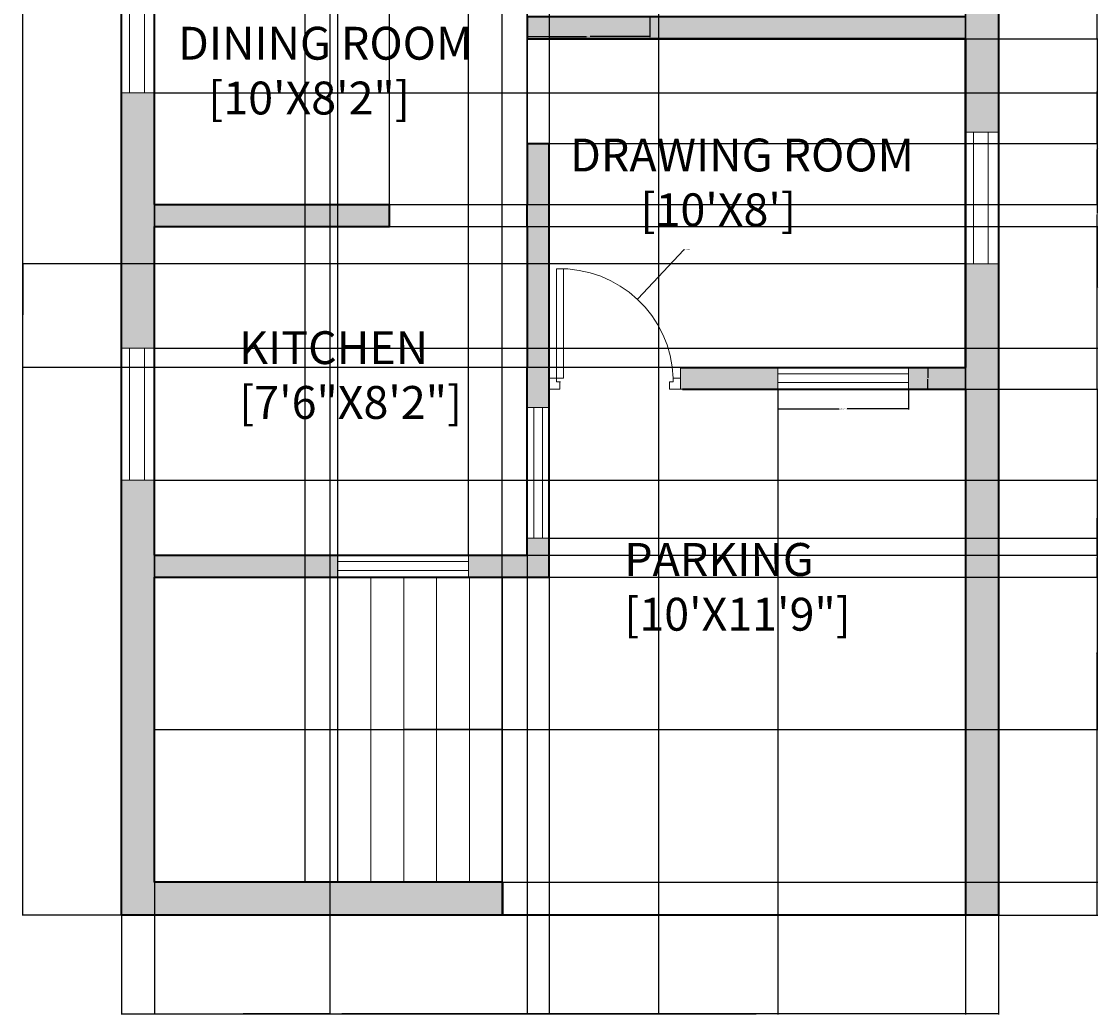
# Model space of a CAD drawing. Units: inches. Extents: x 1963 to 2258, y 1522 to 2116.
# Tile 1 of 3: x 1963 to 2258, y 1522 to 1793. Entities that reach past the tile are written whole.
import ezdxf

# ---------------------------------------------------------------- set-up
doc = ezdxf.new("R2010")
doc.units = ezdxf.units.IN
for name, color, linetype, lineweight in [('A-ANNO-DIMS', 2, 'Continuous', 18), ('A-AREA-IDEN', 7, 'Continuous', 18), ('A-DOOR', 3, 'Continuous', 18), ('A-FLOR-STRS', 7, 'Continuous', 18), ('A-GLAZ', 4, 'Continuous', 18), ('A-WALL', 7, 'Continuous', 35), ('A-WALL-PATT', 250, 'Continuous', 13)]:
    doc.layers.add(name, color=color, linetype=linetype, lineweight=lineweight)
doc.styles.get("Standard").update_dxf_attribs({"font": 'arial.ttf'})
doc.dimstyles.get("Standard").update_dxf_attribs({"dimtxt": 0.18, "dimasz": 0.18, "dimexe": 0.18, "dimexo": 0.0625, "dimgap": 0.09, "dimtad": 0, "dimtih": 1, "dimtoh": 1, "dimdec": 4, "dimzin": 0, "dimdsep": 46, "dimtxsty": 'Standard', "dimcen": 0.09, "dimadec": 0, "dimazin": 0, "dimtfac": 1, "dimtdec": 4, "dimtofl": 0, "dimtmove": 0, "dimatfit": 3, "dimfxl": 1, "dimtolj": 1, "dimtzin": 0, "dimarcsym": 0})

# ---------------------------------------------------------------- blocks, each defined once
blk = doc.blocks.new('WIN-36-9IN-WALL')
for p, q in [((-9, 0), (-9, 36.12)), ((-9, 36.12), (0, 36.12)), ((-6.81, 0), (-6.81, 36.12)), ((-4.5, 36.12), (-2.78, 36.12)), ((-2.78, 36.12), (-2.78, 0)), ((0, 36.12), (0, 0)), ((0, 0), (-9, 0)), ((-2.78, 0), (-6.81, 0)), ((0, 0), (-4.5, 0))]:
    blk.add_line(p, q)
blk = doc.blocks.new('WIN-36-6IN-WALL')
for p, q in [((35.74, 5.97), (0, 5.97)), ((0, 5.97), (0, 0)), ((35.74, 0), (35.74, 5.97)), ((0, 1.82), (0, 4.22)), ((0, 4.22), (35.74, 4.22)), ((0, 0), (0, 2.99)), ((35.74, 2.99), (35.74, 4.22)), ((35.74, 4.22), (35.74, 1.82)), ((35.74, 1.82), (0, 1.82)), ((0, 0), (35.74, 0))]:
    blk.add_line(p, q)
blk = doc.blocks.new('*D8')
at = {"layer": 'A-ANNO-DIMS', "color": 0, "lineweight": -2, "transparency": 16777216}
for p, q in [((2169.76, 1692.68), (2169.76, 1687.21)), ((2205.49, 1692.68), (2205.49, 1687.21)), ((2169.94, 1687.39), (2186.51, 1687.39)), ((2205.31, 1687.39), (2188.74, 1687.39))]:
    blk.add_line(p, q, dxfattribs=at)
at = {"layer": 'A-ANNO-DIMS', "color": 0, "transparency": 16777216}
for points in [[(2169.94, 1687.42), (2169.94, 1687.36), (2169.76, 1687.39)], [(2205.31, 1687.42), (2205.31, 1687.36), (2205.49, 1687.39)]]:
    blk.add_solid(points, dxfattribs=at)
at = {"layer": 'Defpoints', "color": 0, "transparency": 16777216}
for p in [(2169.76, 1692.75), (2205.49, 1692.75), (2205.49, 1687.39)]:
    blk.add_point(p, dxfattribs=at)
at = {"layer": 'A-ANNO-DIMS', "color": 0, "transparency": 16777216, "insert": (2187.62, 1687.39), "char_height": 0.18, "attachment_point": 5}
blk.add_mtext('\\A1;WINDOW 36 TYP.', dxfattribs=at)
blk = doc.blocks.new('*D9')
at = {"layer": 'A-ANNO-DIMS', "color": 0, "lineweight": -2, "transparency": 16777216}
for p, q in [((2205.56, 1698.72), (2211.03, 1698.72)), ((2210.85, 1698.54), (2210.85, 1695.92)), ((2210.85, 1692.93), (2210.85, 1695.55)), ((2205.56, 1692.75), (2211.03, 1692.75))]:
    blk.add_line(p, q, dxfattribs=at)
at = {"layer": 'A-ANNO-DIMS', "color": 0, "transparency": 16777216}
for points in [[(2210.82, 1698.54), (2210.88, 1698.54), (2210.85, 1698.72)], [(2210.82, 1692.93), (2210.88, 1692.93), (2210.85, 1692.75)]]:
    blk.add_solid(points, dxfattribs=at)
at = {"layer": 'Defpoints', "color": 0, "transparency": 16777216}
for p in [(2205.49, 1698.72), (2210.85, 1698.72), (2205.49, 1692.75)]:
    blk.add_point(p, dxfattribs=at)
at = {"layer": 'A-ANNO-DIMS', "color": 0, "transparency": 16777216, "insert": (2210.85, 1695.73), "char_height": 0.18, "attachment_point": 5}
blk.add_mtext('\\A1;6 TYP.', dxfattribs=at)
blk = doc.blocks.new('*D13')
at = {"layer": 'A-ANNO-DIMS', "color": 0, "lineweight": -2, "transparency": 16777216}
for p, q in [((2101.11, 1794.68), (2101.11, 1789.17)), ((2134.66, 1794.68), (2134.66, 1789.17)), ((2101.29, 1789.35), (2117.36, 1789.35)), ((2134.48, 1789.35), (2118.41, 1789.35))]:
    blk.add_line(p, q, dxfattribs=at)
at = {"layer": 'A-ANNO-DIMS', "color": 0, "transparency": 16777216}
for points in [[(2101.29, 1789.38), (2101.29, 1789.32), (2101.11, 1789.35)], [(2134.48, 1789.38), (2134.48, 1789.32), (2134.66, 1789.35)]]:
    blk.add_solid(points, dxfattribs=at)
at = {"layer": 'Defpoints', "color": 0, "transparency": 16777216}
for p in [(2101.11, 1794.75), (2134.66, 1794.75), (2134.66, 1789.35)]:
    blk.add_point(p, dxfattribs=at)
at = {"layer": 'A-ANNO-DIMS', "color": 0, "transparency": 16777216, "insert": (2117.89, 1789.35), "char_height": 0.18, "attachment_point": 5}
blk.add_mtext('\\A1;34 TYP.', dxfattribs=at)
blk = doc.blocks.new('*D14')
at = {"layer": 'A-ANNO-DIMS', "color": 0, "lineweight": -2, "transparency": 16777216}
for p, q in [((1990.11, 1548.68), (1990.11, 1521.53)), ((2230.11, 1548.68), (2230.11, 1521.53)), ((1990.29, 1521.71), (2109.82, 1521.71)), ((2229.93, 1521.71), (2110.4, 1521.71))]:
    blk.add_line(p, q, dxfattribs=at)
at = {"layer": 'A-ANNO-DIMS', "color": 0, "transparency": 16777216}
for points in [[(1990.29, 1521.74), (1990.29, 1521.68), (1990.11, 1521.71)], [(2229.93, 1521.74), (2229.93, 1521.68), (2230.11, 1521.71)]]:
    blk.add_solid(points, dxfattribs=at)
at = {"layer": 'Defpoints', "color": 0, "transparency": 16777216}
for p in [(1990.11, 1548.75), (2230.11, 1548.75), (2230.11, 1521.71)]:
    blk.add_point(p, dxfattribs=at)
at = {"layer": 'A-ANNO-DIMS', "color": 0, "transparency": 16777216, "insert": (2110.11, 1521.71), "char_height": 0.18, "attachment_point": 5}
blk.add_mtext('\\A1;240', dxfattribs=at)
blk = doc.blocks.new('*D15')
at = {"layer": 'A-ANNO-DIMS', "color": 0, "lineweight": -2, "transparency": 16777216}
for p, q in [((2094.32, 1548.81), (2094.32, 2115.96)), ((2094.5, 2115.78), (2157.26, 2115.78)), ((2220.93, 2115.78), (2158.17, 2115.78)), ((2221.11, 1548.81), (2221.11, 2115.96))]:
    blk.add_line(p, q, dxfattribs=at)
at = {"layer": 'A-ANNO-DIMS', "color": 0, "transparency": 16777216}
for points in [[(2094.5, 2115.81), (2094.5, 2115.75), (2094.32, 2115.78)], [(2220.93, 2115.81), (2220.93, 2115.75), (2221.11, 2115.78)]]:
    blk.add_solid(points, dxfattribs=at)
at = {"layer": 'Defpoints', "color": 0, "transparency": 16777216}
for p in [(2221.11, 2115.78), (2094.32, 1548.75), (2221.11, 1548.75)]:
    blk.add_point(p, dxfattribs=at)
at = {"layer": 'A-ANNO-DIMS', "color": 0, "transparency": 16777216, "insert": (2157.72, 2115.78), "char_height": 0.18, "attachment_point": 5}
blk.add_mtext('\\A1;126.79', dxfattribs=at)
blk = doc.blocks.new('*D18')
at = {"layer": 'A-ANNO-DIMS', "color": 0, "lineweight": -2, "transparency": 16777216}
for p, q in [((1999.11, 2079.68), (1999.11, 1521.53)), ((2101.11, 2079.68), (2101.11, 1521.53)), ((1999.29, 1521.71), (2049.83, 1521.71)), ((2100.93, 1521.71), (2050.39, 1521.71))]:
    blk.add_line(p, q, dxfattribs=at)
at = {"layer": 'A-ANNO-DIMS', "color": 0, "transparency": 16777216}
for points in [[(1999.29, 1521.74), (1999.29, 1521.68), (1999.11, 1521.71)], [(2100.93, 1521.74), (2100.93, 1521.68), (2101.11, 1521.71)]]:
    blk.add_solid(points, dxfattribs=at)
at = {"layer": 'Defpoints', "color": 0, "transparency": 16777216}
for p in [(1999.11, 2079.75), (2101.11, 2079.75), (2101.11, 1521.71)]:
    blk.add_point(p, dxfattribs=at)
at = {"layer": 'A-ANNO-DIMS', "color": 0, "transparency": 16777216, "insert": (2050.11, 1521.71), "char_height": 0.18, "attachment_point": 5}
blk.add_mtext('\\A1;102', dxfattribs=at)
blk = doc.blocks.new('*D19')
at = {"layer": 'A-ANNO-DIMS', "color": 0, "lineweight": -2, "transparency": 16777216}
for p, q in [((2094.39, 1641.32), (2257.32, 1641.32)), ((2257.14, 1641.14), (2257.14, 1599.72)), ((2257.14, 1557.93), (2257.14, 1599.35)), ((2094.39, 1557.75), (2257.32, 1557.75))]:
    blk.add_line(p, q, dxfattribs=at)
at = {"layer": 'A-ANNO-DIMS', "color": 0, "transparency": 16777216}
for points in [[(2257.11, 1641.14), (2257.17, 1641.14), (2257.14, 1641.32)], [(2257.11, 1557.93), (2257.17, 1557.93), (2257.14, 1557.75)]]:
    blk.add_solid(points, dxfattribs=at)
at = {"layer": 'Defpoints', "color": 0, "transparency": 16777216}
for p in [(2094.32, 1641.32), (2257.14, 1641.32), (2094.32, 1557.75)]:
    blk.add_point(p, dxfattribs=at)
at = {"layer": 'A-ANNO-DIMS', "color": 0, "transparency": 16777216, "insert": (2257.14, 1599.53), "char_height": 0.18, "attachment_point": 5}
blk.add_mtext('\\A1;83.57', dxfattribs=at)
blk = doc.blocks.new('*D20')
at = {"layer": 'A-ANNO-DIMS', "color": 0, "lineweight": -2, "transparency": 16777216}
for p, q in [((1999.17, 1667.87), (2257.32, 1667.87)), ((2257.14, 1667.69), (2257.14, 1657.77)), ((2257.14, 1647.5), (2257.14, 1657.41)), ((1999.17, 1647.32), (2257.32, 1647.32))]:
    blk.add_line(p, q, dxfattribs=at)
at = {"layer": 'A-ANNO-DIMS', "color": 0, "transparency": 16777216}
for points in [[(2257.11, 1667.69), (2257.17, 1667.69), (2257.14, 1667.87)], [(2257.11, 1647.5), (2257.17, 1647.5), (2257.14, 1647.32)]]:
    blk.add_solid(points, dxfattribs=at)
at = {"layer": 'Defpoints', "color": 0, "transparency": 16777216}
for p in [(1999.11, 1667.87), (2257.14, 1667.87), (1999.11, 1647.32)]:
    blk.add_point(p, dxfattribs=at)
at = {"layer": 'A-ANNO-DIMS', "color": 0, "transparency": 16777216, "insert": (2257.14, 1657.59), "char_height": 0.18, "attachment_point": 5}
blk.add_mtext('\\A1;20.545', dxfattribs=at)
blk = doc.blocks.new('*D21')
at = {"layer": 'A-ANNO-DIMS', "color": 0, "lineweight": -2, "transparency": 16777216}
for p, q in [((1999.17, 1737.32), (2257.32, 1737.32)), ((2257.14, 1737.14), (2257.14, 1720.83)), ((2257.14, 1704.17), (2257.14, 1720.47)), ((1999.17, 1703.99), (2257.32, 1703.99))]:
    blk.add_line(p, q, dxfattribs=at)
at = {"layer": 'A-ANNO-DIMS', "color": 0, "transparency": 16777216}
for points in [[(2257.11, 1737.14), (2257.17, 1737.14), (2257.14, 1737.32)], [(2257.11, 1704.17), (2257.17, 1704.17), (2257.14, 1703.99)]]:
    blk.add_solid(points, dxfattribs=at)
at = {"layer": 'Defpoints', "color": 0, "transparency": 16777216}
for p in [(1999.11, 1737.32), (2257.14, 1737.32), (1999.11, 1703.99)]:
    blk.add_point(p, dxfattribs=at)
at = {"layer": 'A-ANNO-DIMS', "color": 0, "transparency": 16777216, "insert": (2257.14, 1720.65), "char_height": 0.18, "attachment_point": 5}
blk.add_mtext('\\A1;33.334', dxfattribs=at)
blk = doc.blocks.new('*D22')
at = {"layer": 'A-ANNO-DIMS', "color": 0, "lineweight": -2, "transparency": 16777216}
for p, q in [((1999.17, 1773.95), (2257.32, 1773.95)), ((2257.14, 1773.77), (2257.14, 1758.82)), ((2257.14, 1743.5), (2257.14, 1758.45)), ((1999.17, 1743.32), (2257.32, 1743.32))]:
    blk.add_line(p, q, dxfattribs=at)
at = {"layer": 'A-ANNO-DIMS', "color": 0, "transparency": 16777216}
for points in [[(2257.11, 1773.77), (2257.17, 1773.77), (2257.14, 1773.95)], [(2257.11, 1743.5), (2257.17, 1743.5), (2257.14, 1743.32)]]:
    blk.add_solid(points, dxfattribs=at)
at = {"layer": 'Defpoints', "color": 0, "transparency": 16777216}
for p in [(1999.11, 1773.95), (2257.14, 1773.95), (1999.11, 1743.32)]:
    blk.add_point(p, dxfattribs=at)
at = {"layer": 'A-ANNO-DIMS', "color": 0, "transparency": 16777216, "insert": (2257.14, 1758.64), "char_height": 0.18, "attachment_point": 5}
blk.add_mtext('\\A1;30.634', dxfattribs=at)
blk = doc.blocks.new('*D26')
at = {"layer": 'A-ANNO-DIMS', "color": 0, "lineweight": -2, "transparency": 16777216}
for p, q in [((2221.17, 1692.75), (2257.32, 1692.75)), ((2257.14, 1692.57), (2257.14, 1620.93)), ((2257.14, 1548.93), (2257.14, 1620.57)), ((2230.17, 1548.75), (2257.32, 1548.75))]:
    blk.add_line(p, q, dxfattribs=at)
at = {"layer": 'A-ANNO-DIMS', "color": 0, "transparency": 16777216}
for points in [[(2257.11, 1692.57), (2257.17, 1692.57), (2257.14, 1692.75)], [(2257.11, 1548.93), (2257.17, 1548.93), (2257.14, 1548.75)]]:
    blk.add_solid(points, dxfattribs=at)
at = {"layer": 'Defpoints', "color": 0, "transparency": 16777216}
for p in [(2221.11, 1692.75), (2257.14, 1692.75), (2230.11, 1548.75)]:
    blk.add_point(p, dxfattribs=at)
at = {"layer": 'A-ANNO-DIMS', "color": 0, "transparency": 16777216, "insert": (2257.14, 1620.75), "char_height": 0.18, "attachment_point": 5}
blk.add_mtext('\\A1;144', dxfattribs=at)
blk = doc.blocks.new('*D27')
at = {"layer": 'A-ANNO-DIMS', "color": 0, "lineweight": -2, "transparency": 16777216}
for p, q in [((2221.17, 1788.75), (2257.32, 1788.75)), ((2257.14, 1788.57), (2257.14, 1740.93)), ((2257.14, 1692.93), (2257.14, 1740.57)), ((2221.17, 1692.75), (2257.32, 1692.75))]:
    blk.add_line(p, q, dxfattribs=at)
at = {"layer": 'A-ANNO-DIMS', "color": 0, "transparency": 16777216}
for points in [[(2257.11, 1788.57), (2257.17, 1788.57), (2257.14, 1788.75)], [(2257.11, 1692.93), (2257.17, 1692.93), (2257.14, 1692.75)]]:
    blk.add_solid(points, dxfattribs=at)
at = {"layer": 'Defpoints', "color": 0, "transparency": 16777216}
for p in [(2221.11, 1788.75), (2257.14, 1788.75), (2221.11, 1692.75)]:
    blk.add_point(p, dxfattribs=at)
at = {"layer": 'A-ANNO-DIMS', "color": 0, "transparency": 16777216, "insert": (2257.14, 1740.75), "char_height": 0.18, "attachment_point": 5}
blk.add_mtext('\\A1;96', dxfattribs=at)
blk = doc.blocks.new('*D28')
at = {"layer": 'A-ANNO-DIMS', "color": 0, "lineweight": -2, "transparency": 16777216}
for p, q in [((2221.17, 1896.75), (2257.32, 1896.75)), ((2257.14, 1896.57), (2257.14, 1842.93)), ((2257.14, 1788.93), (2257.14, 1842.57)), ((2221.17, 1788.75), (2257.32, 1788.75))]:
    blk.add_line(p, q, dxfattribs=at)
at = {"layer": 'A-ANNO-DIMS', "color": 0, "transparency": 16777216}
for points in [[(2257.11, 1896.57), (2257.17, 1896.57), (2257.14, 1896.75)], [(2257.11, 1788.93), (2257.17, 1788.93), (2257.14, 1788.75)]]:
    blk.add_solid(points, dxfattribs=at)
at = {"layer": 'Defpoints', "color": 0, "transparency": 16777216}
for p in [(2221.11, 1896.75), (2257.14, 1896.75), (2221.11, 1788.75)]:
    blk.add_point(p, dxfattribs=at)
at = {"layer": 'A-ANNO-DIMS', "color": 0, "transparency": 16777216, "insert": (2257.14, 1842.75), "char_height": 0.18, "attachment_point": 5}
blk.add_mtext('\\A1;108', dxfattribs=at)
blk = doc.blocks.new('*D30')
at = {"layer": 'A-ANNO-DIMS', "color": 0, "lineweight": -2, "transparency": 16777216}
for p, q in [((2221.05, 1727.08), (1962.89, 1727.08)), ((1963.07, 1726.9), (1963.07, 1713.1)), ((1963.07, 1698.93), (1963.07, 1712.73)), ((2221.05, 1698.75), (1962.89, 1698.75))]:
    blk.add_line(p, q, dxfattribs=at)
at = {"layer": 'A-ANNO-DIMS', "color": 0, "transparency": 16777216}
for points in [[(1963.04, 1726.9), (1963.1, 1726.9), (1963.07, 1727.08)], [(1963.04, 1698.93), (1963.1, 1698.93), (1963.07, 1698.75)]]:
    blk.add_solid(points, dxfattribs=at)
at = {"layer": 'Defpoints', "color": 0, "transparency": 16777216}
for p in [(2221.11, 1727.08), (1963.07, 1698.75), (2221.11, 1698.75)]:
    blk.add_point(p, dxfattribs=at)
at = {"layer": 'A-ANNO-DIMS', "color": 0, "transparency": 16777216, "insert": (1963.07, 1712.91), "char_height": 0.18, "attachment_point": 5}
blk.add_mtext('\\A1;28.334', dxfattribs=at)
blk = doc.blocks.new('*D33')
at = {"layer": 'A-ANNO-DIMS', "color": 0, "lineweight": -2, "transparency": 16777216}
for p, q in [((1999.11, 1863.26), (1999.11, 1521.53)), ((2047.11, 1863.26), (2047.11, 1521.53)), ((1999.29, 1521.71), (2022.89, 1521.71)), ((2046.93, 1521.71), (2023.33, 1521.71))]:
    blk.add_line(p, q, dxfattribs=at)
at = {"layer": 'A-ANNO-DIMS', "color": 0, "transparency": 16777216}
for points in [[(1999.29, 1521.74), (1999.29, 1521.68), (1999.11, 1521.71)], [(2046.93, 1521.74), (2046.93, 1521.68), (2047.11, 1521.71)]]:
    blk.add_solid(points, dxfattribs=at)
at = {"layer": 'Defpoints', "color": 0, "transparency": 16777216}
for p in [(1999.11, 1863.32), (2047.11, 1863.32), (2047.11, 1521.71)]:
    blk.add_point(p, dxfattribs=at)
at = {"layer": 'A-ANNO-DIMS', "color": 0, "transparency": 16777216, "insert": (2023.11, 1521.71), "char_height": 0.18, "attachment_point": 5}
blk.add_mtext('\\A1;48', dxfattribs=at)
blk = doc.blocks.new('*D34')
at = {"layer": 'A-ANNO-DIMS', "color": 0, "lineweight": -2, "transparency": 16777216}
for p, q in [((2047.11, 1971.68), (2047.11, 1521.53)), ((2137.11, 1971.68), (2137.11, 1521.53)), ((2047.29, 1521.71), (2091.89, 1521.71)), ((2136.93, 1521.71), (2092.33, 1521.71))]:
    blk.add_line(p, q, dxfattribs=at)
at = {"layer": 'A-ANNO-DIMS', "color": 0, "transparency": 16777216}
for points in [[(2047.29, 1521.74), (2047.29, 1521.68), (2047.11, 1521.71)], [(2136.93, 1521.74), (2136.93, 1521.68), (2137.11, 1521.71)]]:
    blk.add_solid(points, dxfattribs=at)
at = {"layer": 'Defpoints', "color": 0, "transparency": 16777216}
for p in [(2047.11, 1971.75), (2137.11, 1971.75), (2137.11, 1521.71)]:
    blk.add_point(p, dxfattribs=at)
at = {"layer": 'A-ANNO-DIMS', "color": 0, "transparency": 16777216, "insert": (2092.11, 1521.71), "char_height": 0.18, "attachment_point": 5}
blk.add_mtext('\\A1;90', dxfattribs=at)
blk = doc.blocks.new('*D37')
at = {"layer": 'A-ANNO-DIMS', "color": 0, "lineweight": -2, "transparency": 16777216}
for p, q in [((1999.11, 1743.38), (1999.11, 2115.96)), ((1999.29, 2115.78), (2030.89, 2115.78)), ((2063.27, 2115.78), (2031.67, 2115.78)), ((2063.45, 1743.38), (2063.45, 2115.96))]:
    blk.add_line(p, q, dxfattribs=at)
at = {"layer": 'A-ANNO-DIMS', "color": 0, "transparency": 16777216}
for points in [[(1999.29, 2115.81), (1999.29, 2115.75), (1999.11, 2115.78)], [(2063.27, 2115.81), (2063.27, 2115.75), (2063.45, 2115.78)]]:
    blk.add_solid(points, dxfattribs=at)
at = {"layer": 'Defpoints', "color": 0, "transparency": 16777216}
for p in [(2063.45, 2115.78), (1999.11, 1743.32), (2063.45, 1743.32)]:
    blk.add_point(p, dxfattribs=at)
at = {"layer": 'A-ANNO-DIMS', "color": 0, "transparency": 16777216, "insert": (2031.28, 2115.78), "char_height": 0.18, "attachment_point": 5}
blk.add_mtext('\\A1;64.34', dxfattribs=at)
blk = doc.blocks.new('*D38')
at = {"layer": 'A-ANNO-DIMS', "color": 0, "lineweight": -2, "transparency": 16777216}
for p, q in [((1999.11, 1647.38), (1999.11, 2115.96)), ((1999.29, 2115.78), (2023.84, 2115.78)), ((2049.14, 2115.78), (2024.59, 2115.78)), ((2049.32, 1647.35), (2049.32, 2115.96))]:
    blk.add_line(p, q, dxfattribs=at)
at = {"layer": 'A-ANNO-DIMS', "color": 0, "transparency": 16777216}
for points in [[(1999.29, 2115.81), (1999.29, 2115.75), (1999.11, 2115.78)], [(2049.14, 2115.81), (2049.14, 2115.75), (2049.32, 2115.78)]]:
    blk.add_solid(points, dxfattribs=at)
at = {"layer": 'Defpoints', "color": 0, "transparency": 16777216}
for p in [(2049.32, 2115.78), (1999.11, 1647.32), (2049.32, 1647.29)]:
    blk.add_point(p, dxfattribs=at)
at = {"layer": 'A-ANNO-DIMS', "color": 0, "transparency": 16777216, "insert": (2024.22, 2115.78), "char_height": 0.18, "attachment_point": 5}
blk.add_mtext('\\A1;50.21', dxfattribs=at)
blk = doc.blocks.new('*D39')
at = {"layer": 'A-ANNO-DIMS', "color": 0, "lineweight": -2, "transparency": 16777216}
for p, q in [((2107.11, 1692.68), (2107.11, 1521.53)), ((2169.76, 1692.68), (2169.76, 1521.53)), ((2107.29, 1521.71), (2138.04, 1521.71)), ((2169.58, 1521.71), (2138.83, 1521.71))]:
    blk.add_line(p, q, dxfattribs=at)
at = {"layer": 'A-ANNO-DIMS', "color": 0, "transparency": 16777216}
for points in [[(2107.29, 1521.74), (2107.29, 1521.68), (2107.11, 1521.71)], [(2169.58, 1521.74), (2169.58, 1521.68), (2169.76, 1521.71)]]:
    blk.add_solid(points, dxfattribs=at)
at = {"layer": 'Defpoints', "color": 0, "transparency": 16777216}
for p in [(2107.11, 1692.75), (2169.76, 1692.75), (2169.76, 1521.71)]:
    blk.add_point(p, dxfattribs=at)
at = {"layer": 'A-ANNO-DIMS', "color": 0, "transparency": 16777216, "insert": (2138.43, 1521.71), "char_height": 0.18, "attachment_point": 5}
blk.add_mtext('\\A1;62.65', dxfattribs=at)
blk = doc.blocks.new('*D40')
at = {"layer": 'A-ANNO-DIMS', "color": 0, "lineweight": -2, "transparency": 16777216}
for p, q in [((2107.17, 1652), (2257.32, 1652)), ((2257.14, 1651.82), (2257.14, 1646.84)), ((2257.14, 1641.5), (2257.14, 1646.48)), ((2107.17, 1641.32), (2257.32, 1641.32))]:
    blk.add_line(p, q, dxfattribs=at)
at = {"layer": 'A-ANNO-DIMS', "color": 0, "transparency": 16777216}
for points in [[(2257.11, 1651.82), (2257.17, 1651.82), (2257.14, 1652)], [(2257.11, 1641.5), (2257.17, 1641.5), (2257.14, 1641.32)]]:
    blk.add_solid(points, dxfattribs=at)
at = {"layer": 'Defpoints', "color": 0, "transparency": 16777216}
for p in [(2107.11, 1652), (2257.14, 1652), (2107.11, 1641.32)]:
    blk.add_point(p, dxfattribs=at)
at = {"layer": 'A-ANNO-DIMS', "color": 0, "transparency": 16777216, "insert": (2257.14, 1646.66), "char_height": 0.18, "attachment_point": 5}
blk.add_mtext('\\A1;10.683', dxfattribs=at)
blk = doc.blocks.new('*D41')
at = {"layer": 'A-ANNO-DIMS', "color": 0, "lineweight": -2, "transparency": 16777216}
for p, q in [((2101.17, 1788.75), (2257.32, 1788.75)), ((2257.14, 1788.57), (2257.14, 1774.6)), ((2257.14, 1760.27), (2257.14, 1774.24)), ((2101.17, 1760.09), (2257.32, 1760.09))]:
    blk.add_line(p, q, dxfattribs=at)
at = {"layer": 'A-ANNO-DIMS', "color": 0, "transparency": 16777216}
for points in [[(2257.11, 1788.57), (2257.17, 1788.57), (2257.14, 1788.75)], [(2257.11, 1760.27), (2257.17, 1760.27), (2257.14, 1760.09)]]:
    blk.add_solid(points, dxfattribs=at)
at = {"layer": 'Defpoints', "color": 0, "transparency": 16777216}
for p in [(2101.11, 1788.75), (2257.14, 1788.75), (2101.11, 1760.09)]:
    blk.add_point(p, dxfattribs=at)
at = {"layer": 'A-ANNO-DIMS', "color": 0, "transparency": 16777216, "insert": (2257.14, 1774.42), "char_height": 0.18, "attachment_point": 5}
blk.add_mtext('\\A1;28.66', dxfattribs=at)
blk = doc.blocks.new('*D42')
at = {"layer": 'A-ANNO-DIMS', "color": 0, "lineweight": -2, "transparency": 16777216}
for p, q in [((1999.11, 1557.81), (1999.11, 2115.96)), ((1999.29, 2115.78), (2019.25, 2115.78)), ((2040.14, 2115.78), (2020.18, 2115.78)), ((2040.32, 1557.81), (2040.32, 2115.96))]:
    blk.add_line(p, q, dxfattribs=at)
at = {"layer": 'A-ANNO-DIMS', "color": 0, "transparency": 16777216}
for points in [[(1999.29, 2115.81), (1999.29, 2115.75), (1999.11, 2115.78)], [(2040.14, 2115.81), (2040.14, 2115.75), (2040.32, 2115.78)]]:
    blk.add_solid(points, dxfattribs=at)
at = {"layer": 'Defpoints', "color": 0, "transparency": 16777216}
for p in [(2040.32, 2115.78), (1999.11, 1557.75), (2040.32, 1557.75)]:
    blk.add_point(p, dxfattribs=at)
at = {"layer": 'A-ANNO-DIMS', "color": 0, "transparency": 16777216, "insert": (2019.72, 2115.78), "char_height": 0.18, "attachment_point": 5}
blk.add_mtext('\\A1;41.214', dxfattribs=at)
blk = doc.blocks.new('*D43')
at = {"layer": 'A-ANNO-DIMS', "color": 0, "lineweight": -2, "transparency": 16777216}
for p, q in [((2040.32, 1557.81), (2040.32, 2115.96)), ((2040.5, 2115.78), (2044.67, 2115.78)), ((2049.14, 2115.78), (2044.97, 2115.78)), ((2049.32, 1557.81), (2049.32, 2115.96))]:
    blk.add_line(p, q, dxfattribs=at)
at = {"layer": 'A-ANNO-DIMS', "color": 0, "transparency": 16777216}
for points in [[(2040.5, 2115.81), (2040.5, 2115.75), (2040.32, 2115.78)], [(2049.14, 2115.81), (2049.14, 2115.75), (2049.32, 2115.78)]]:
    blk.add_solid(points, dxfattribs=at)
at = {"layer": 'Defpoints', "color": 0, "transparency": 16777216}
for p in [(2049.32, 2115.78), (2040.32, 1557.75), (2049.32, 1557.75)]:
    blk.add_point(p, dxfattribs=at)
at = {"layer": 'A-ANNO-DIMS', "color": 0, "transparency": 16777216, "insert": (2044.82, 2115.78), "char_height": 0.18, "attachment_point": 5}
blk.add_mtext('\\A1;9', dxfattribs=at)
blk = doc.blocks.new('*D44')
at = {"layer": 'A-ANNO-DIMS', "color": 0, "lineweight": -2, "transparency": 16777216}
for p, q in [((1999.17, 1641.32), (2257.32, 1641.32)), ((2257.14, 1641.14), (2257.14, 1620.61)), ((2257.14, 1599.71), (2257.14, 1620.24)), ((1999.17, 1599.53), (2257.32, 1599.53))]:
    blk.add_line(p, q, dxfattribs=at)
at = {"layer": 'A-ANNO-DIMS', "color": 0, "transparency": 16777216}
for points in [[(2257.11, 1641.14), (2257.17, 1641.14), (2257.14, 1641.32)], [(2257.11, 1599.71), (2257.17, 1599.71), (2257.14, 1599.53)]]:
    blk.add_solid(points, dxfattribs=at)
at = {"layer": 'Defpoints', "color": 0, "transparency": 16777216}
for p in [(1999.11, 1641.32), (2257.14, 1641.32), (1999.11, 1599.53)]:
    blk.add_point(p, dxfattribs=at)
at = {"layer": 'A-ANNO-DIMS', "color": 0, "transparency": 16777216, "insert": (2257.14, 1620.43), "char_height": 0.18, "attachment_point": 5}
blk.add_mtext('\\A1;41.79', dxfattribs=at)
blk = doc.blocks.new('*D45')
at = {"layer": 'A-ANNO-DIMS', "color": 0, "lineweight": -2, "transparency": 16777216}
for p, q in [((2107.11, 1896.68), (2107.11, 1521.53)), ((2221.11, 1896.68), (2221.11, 1521.53)), ((2107.29, 1521.71), (2163.83, 1521.71)), ((2220.93, 1521.71), (2164.39, 1521.71))]:
    blk.add_line(p, q, dxfattribs=at)
at = {"layer": 'A-ANNO-DIMS', "color": 0, "transparency": 16777216}
for points in [[(2107.29, 1521.74), (2107.29, 1521.68), (2107.11, 1521.71)], [(2220.93, 1521.74), (2220.93, 1521.68), (2221.11, 1521.71)]]:
    blk.add_solid(points, dxfattribs=at)
at = {"layer": 'Defpoints', "color": 0, "transparency": 16777216}
for p in [(2107.11, 1896.75), (2221.11, 1896.75), (2221.11, 1521.71)]:
    blk.add_point(p, dxfattribs=at)
at = {"layer": 'A-ANNO-DIMS', "color": 0, "transparency": 16777216, "insert": (2164.11, 1521.71), "char_height": 0.18, "attachment_point": 5}
blk.add_mtext('\\A1;114', dxfattribs=at)
blk = doc.blocks.new('*D46')
at = {"layer": 'A-ANNO-DIMS', "color": 0, "lineweight": -2, "transparency": 16777216}
for p, q in [((2085.06, 1647.35), (2085.06, 2115.96)), ((2085.24, 2115.78), (2092.7, 2115.78)), ((2100.93, 2115.78), (2093.47, 2115.78)), ((2101.11, 1647.38), (2101.11, 2115.96))]:
    blk.add_line(p, q, dxfattribs=at)
at = {"layer": 'A-ANNO-DIMS', "color": 0, "transparency": 16777216}
for points in [[(2085.24, 2115.81), (2085.24, 2115.75), (2085.06, 2115.78)], [(2100.93, 2115.81), (2100.93, 2115.75), (2101.11, 2115.78)]]:
    blk.add_solid(points, dxfattribs=at)
at = {"layer": 'Defpoints', "color": 0, "transparency": 16777216}
for p in [(2101.11, 2115.78), (2085.06, 1647.29), (2101.11, 1647.32)]:
    blk.add_point(p, dxfattribs=at)
at = {"layer": 'A-ANNO-DIMS', "color": 0, "transparency": 16777216, "insert": (2093.08, 2115.78), "char_height": 0.18, "attachment_point": 5}
blk.add_mtext('\\A1;16.05', dxfattribs=at)
blk = doc.blocks.new('*D47')
at = {"layer": 'A-ANNO-DIMS', "color": 0, "lineweight": -2, "transparency": 16777216}
for p, q in [((1990.05, 2088.75), (1962.89, 2088.75)), ((1963.07, 2088.57), (1963.07, 1818.93)), ((1963.07, 1548.93), (1963.07, 1818.57)), ((1990.05, 1548.75), (1962.89, 1548.75))]:
    blk.add_line(p, q, dxfattribs=at)
at = {"layer": 'A-ANNO-DIMS', "color": 0, "transparency": 16777216}
for points in [[(1963.04, 2088.57), (1963.1, 2088.57), (1963.07, 2088.75)], [(1963.04, 1548.93), (1963.1, 1548.93), (1963.07, 1548.75)]]:
    blk.add_solid(points, dxfattribs=at)
at = {"layer": 'Defpoints', "color": 0, "transparency": 16777216}
for p in [(1963.07, 2088.75), (1990.11, 2088.75), (1990.11, 1548.75)]:
    blk.add_point(p, dxfattribs=at)
at = {"layer": 'A-ANNO-DIMS', "color": 0, "transparency": 16777216, "insert": (1963.07, 1818.75), "char_height": 0.18, "attachment_point": 5}
blk.add_mtext('\\A1;540', dxfattribs=at)
blk = doc.blocks.new('*D48')
at = {"layer": 'A-ANNO-DIMS', "color": 0, "lineweight": -2, "transparency": 16777216}
for p, q in [((2144.05, 1730.95), (2131.45, 1717.51)), ((2144.23, 1730.95), (2144.05, 1730.95)), ((2110.02, 1694.75), (2110.2, 1694.75)), ((2110.11, 1694.66), (2110.11, 1694.84))]:
    blk.add_line(p, q, dxfattribs=at)
at = {"layer": 'A-ANNO-DIMS', "color": 0, "transparency": 16777216}
blk.add_solid([(2131.42, 1717.53), (2131.47, 1717.49), (2131.32, 1717.38)], dxfattribs=at)
at = {"layer": 'Defpoints', "color": 0, "transparency": 16777216}
for p in [(2131.32, 1717.38), (2110.11, 1694.75)]:
    blk.add_point(p, dxfattribs=at)
at = {"layer": 'A-ANNO-DIMS', "color": 0, "transparency": 16777216, "insert": (2144.97, 1730.95), "char_height": 0.18, "attachment_point": 5}
blk.add_mtext('\\A1;3X R31.016', dxfattribs=at)

msp = doc.modelspace()

# ---------------------------------------------------------------- hatches: boundary and pattern name
at = {"layer": 'A-WALL-PATT'}
h = msp.add_hatch(color=256, dxfattribs=at)
h.dxf.hatch_style = 1
h.paths.add_polyline_path([(2040.4282, 2088.7475), (1990.109, 2088.7475), (1990.109, 2047.2372), (1999.109, 2047.2372), (1999.109, 2079.7475), (2040.4282, 2079.7475)])
h.paths.add_polyline_path([(2159.691, 2088.7475), (2076.5488, 2088.7475), (2076.5488, 2084.2475), (2076.5488, 2079.7475), (2101.109, 2079.7475), (2101.109, 1977.7475), (2101.109, 1971.7475), (2107.109, 1971.7475), (2107.109, 1974.7475), (2107.109, 1977.7475), (2107.109, 2079.7475), (2110.109, 2079.7475), (2159.691, 2079.7475)])
h.paths.add_polyline_path([(2230.109, 2088.7475), (2195.8116, 2088.7475), (2195.8116, 2084.2475), (2195.8116, 2079.7475), (2221.109, 2079.7475), (2221.109, 2045.7556), (2230.109, 2045.7556)])
h.paths.add_polyline_path([(2230.109, 2009.6349), (2225.609, 2009.6349), (2221.109, 2009.6349), (2221.109, 1977.7475), (2173.109, 1977.7475), (2173.109, 1974.7475), (2173.0802, 1971.7475), (2178.9852, 1971.7475), (2185.109, 1971.7475), (2191.109, 1971.7475), (2191.109, 1902.7475), (2143.109, 1902.7475), (2143.109, 1971.7475), (2143.109, 1977.7475), (2137.109, 1977.7475), (2137.109, 1971.7475), (2137.109, 1902.7475), (2101.109, 1902.7475), (2101.109, 1830.7475), (2104.109, 1830.7475), (2107.109, 1830.7475), (2107.109, 1896.7475), (2221.109, 1896.7475), (2221.109, 1871.2465), (2230.109, 1871.2465), (2230.109, 1902.7475), (2197.109, 1902.7475), (2197.109, 1971.7475), (2230.109, 1971.7475)])
h.paths.add_polyline_path([(2065.109, 1977.7475), (1999.109, 1977.7475), (1999.109, 2011.1166), (1994.609, 2011.1166), (1990.109, 2011.1166), (1990.109, 1810.0744), (1999.109, 1810.0744), (1999.109, 1863.32), (2047.109, 1863.32), (2047.109, 1869.32), (2047.109, 1911.4119), (2044.109, 1911.4119), (2041.109, 1911.4119), (2041.109, 1869.32), (1999.109, 1869.32), (1999.109, 1941.32), (2041.109, 1941.32), (2044.109, 1941.32), (2044.109, 1941.4119), (2047.109, 1941.4119), (2047.109, 1971.7475), (2065.109, 1971.7475), (2065.109, 1974.7475)])
h.paths.add_polyline_path([(2041.109, 1971.7475), (2041.109, 1947.32), (1999.109, 1947.32), (1999.109, 1971.7475)], flags=16)
h.paths.add_polyline_path([(2230.109, 1835.1259), (2225.609, 1835.1259), (2221.109, 1835.1259), (2221.109, 1794.7475), (2101.109, 1794.7475), (2101.109, 1788.7475), (2221.109, 1788.7475), (2221.109, 1763.2023), (2230.109, 1763.2023)])
h.paths.add_polyline_path([(2063.4524, 1743.32), (1999.109, 1743.32), (1999.109, 1773.9538), (1994.609, 1773.9538), (1992.3007, 1773.9538), (1990.109, 1773.9538), (1990.109, 1703.9859), (1999.109, 1703.9859), (1999.109, 1737.32), (2063.4524, 1737.32)])
h.paths.add_polyline_path([(2169.7564, 1696.9689), (2169.7564, 1698.7475), (2143.109, 1698.7475), (2143.109, 1692.7475), (2143.6022, 1692.7475), (2169.7564, 1692.7475), (2169.7564, 1695.7336)])
h.paths.add_polyline_path([(2230.109, 1727.0817), (2225.609, 1727.0817), (2221.109, 1727.0817), (2221.109, 1698.7475), (2205.4934, 1698.7475), (2205.4934, 1692.7475), (2221.109, 1692.7475), (2221.109, 1557.7475), (2221.109, 1548.7475), (2230.109, 1548.7475)])
h.paths.add_polyline_path([(2107.109, 1760.0903), (2101.109, 1760.0903), (2101.109, 1743.32), (2101.109, 1737.32), (2101.109, 1698.7475), (2101.109, 1687.7398), (2104.1229, 1687.7398), (2105.3583, 1687.7398), (2107.109, 1687.7398), (2107.109, 1692.7475), (2107.109, 1695.7475), (2107.109, 1698.7475)])
h.paths.add_polyline_path([(2107.109, 1652.0028), (2101.109, 1652.0028), (2101.109, 1647.32), (2085.0601, 1647.32), (2085.0601, 1641.32), (2085.3232, 1641.32), (2107.109, 1641.32)])
h.paths.add_polyline_path([(2049.3232, 1645.5414), (2049.3232, 1647.32), (1999.109, 1647.32), (1999.109, 1667.8653), (1994.609, 1667.8653), (1992.3007, 1667.8653), (1990.109, 1667.8653), (1990.109, 1548.7475), (2094.3232, 1548.7475), (2094.3232, 1557.7475), (2085.3232, 1557.7475), (1999.109, 1557.7475), (1999.109, 1641.32), (2049.3232, 1641.32), (2049.3232, 1644.306)])

# ---------------------------------------------------------------- linework, layer by layer
at = {"layer": 'A-DOOR'}
for p, q in [((2109.109, 1695.7475), (2109.109, 1725.7475)), ((2109.109, 1725.7475), (2111.109, 1725.7475)), ((2111.109, 1725.7475), (2111.109, 1695.7475)), ((2143.109, 1698.7475), (2143.109, 1692.7475)), ((2109.109, 1695.7475), (2107.109, 1695.7475)), ((2107.109, 1695.7475), (2107.109, 1692.7475)), ((2109.109, 1694.7475), (2109.109, 1695.7475)), ((2111.109, 1695.7475), (2109.109, 1695.7475)), ((2141.109, 1694.7475), (2141.109, 1695.7475)), ((2141.109, 1695.7475), (2143.109, 1695.7475)), ((2110.109, 1692.7475), (2107.109, 1692.7475)), ((2110.109, 1694.7475), (2109.109, 1694.7475)), ((2110.109, 1692.7475), (2110.109, 1694.7475)), ((2140.109, 1692.7475), (2140.109, 1694.7475)), ((2140.109, 1694.7475), (2141.109, 1694.7475)), ((2143.109, 1692.7475), (2140.109, 1692.7475)), ((2143.6022, 1692.7475), (2140.6022, 1692.7475)), ((2143.6022, 1692.7475), (2140.6022, 1692.7475))]:
    msp.add_line(p, q, dxfattribs=at)
msp.add_arc((2110.109, 1694.7475), 31.0161, 1.84761, 91.84761, dxfattribs=at)
at = {"layer": 'A-FLOR-STRS'}
for p, q in [((2049.3232, 1641.32), (2040.3232, 1641.32)), ((2040.3232, 1641.32), (2040.3232, 1557.7475)), ((2040.3232, 1599.5337), (2040.3232, 1641.32)), ((2049.3232, 1557.7475), (2049.3232, 1641.32)), ((2067.3232, 1641.32), (2058.3232, 1641.32)), ((2058.3232, 1641.32), (2058.3232, 1557.7475)), ((2067.3232, 1557.7475), (2067.3232, 1641.32)), ((2085.3232, 1641.32), (2076.3232, 1641.32)), ((2076.3232, 1641.32), (2076.3232, 1557.7475)), ((2085.3232, 1557.7475), (2085.3232, 1641.32)), ((2094.3232, 1641.32), (2094.3232, 1557.7475)), ((2040.3232, 1599.5337), (1999.109, 1599.5337)), ((2094.3232, 1599.7475), (2040.3232, 1599.5337)), ((2094.3232, 1557.7475), (2094.3232, 1599.7475)), ((2058.3232, 1557.7475), (2049.3232, 1557.7475)), ((2076.3232, 1557.7475), (2067.3232, 1557.7475)), ((2094.3232, 1557.7475), (2085.3232, 1557.7475))]:
    msp.add_line(p, q, dxfattribs=at)
msp.add_lwpolyline([(2085.3232, 1579.8216, 0, 0, 0), (2019.7161, 1579.8216, 0, 0, 0), (2019.7161, 1620.4269, 0, 0, 0), (2076.3232, 1620.4269, 6, 0, 0), (2094.2413, 1620.4269, 0, 0, 0)], format="xyseb", dxfattribs=at)
at = {"layer": 'A-WALL'}
for p, q in [((1999.109, 1743.32), (1999.109, 1863.32)), ((2221.109, 1788.7475), (2107.109, 1788.7475)), ((2221.109, 1698.7475), (2221.109, 1788.7475)), ((2101.109, 1760.0903), (2107.109, 1760.0903)), ((2101.109, 1760.0903), (2101.109, 1743.32)), ((2107.109, 1698.7475), (2107.109, 1760.0903)), ((1999.109, 1743.32), (2063.4524, 1743.32)), ((2063.4524, 1737.32), (2063.4524, 1743.32)), ((2101.109, 1737.32), (2101.109, 1743.32)), ((1999.109, 1647.32), (1999.109, 1737.32)), ((1999.109, 1737.32), (2063.4524, 1737.32)), ((2101.109, 1737.32), (2101.109, 1698.7475)), ((2101.109, 1647.32), (2101.109, 1698.7475)), ((2107.109, 1692.7475), (2107.109, 1698.7475)), ((2143.109, 1698.7475), (2221.109, 1698.7475)), ((2107.109, 1641.32), (2107.109, 1692.7475)), ((2143.6022, 1692.7475), (2221.109, 1692.7475)), ((1999.109, 1647.32), (2101.109, 1647.32)), ((1999.109, 1557.7475), (1999.109, 1641.32)), ((1999.109, 1641.32), (2107.109, 1641.32)), ((2094.3232, 1557.7475), (2094.3232, 1548.7475)), ((2221.109, 1557.7475), (2221.109, 1548.7475))]:
    msp.add_line(p, q, dxfattribs=at)
for points in [[(1990.109, 2088.7475), (2230.109, 2088.7475), (2230.109, 1548.7475), (1990.109, 1548.7475), (1990.109, 2088.7475)], [(1999.109, 1743.32), (1999.109, 1863.32)], [(2221.109, 1794.7475), (2101.109, 1794.7475), (2101.109, 1788.7475), (2221.109, 1788.7475)], [(2221.109, 1788.7475), (2221.109, 1698.7475)], [(1999.109, 1647.32), (1999.109, 1737.32)], [(2221.109, 1692.7475), (2221.109, 1557.7475)], [(2094.3232, 1557.7475), (1999.109, 1557.7475), (1999.109, 1641.32)]]:
    msp.add_lwpolyline(points, dxfattribs=at)

# ---------------------------------------------------------------- block references
at = {"layer": 'A-GLAZ'}
for name, p in [('WIN-36-9IN-WALL', (1999.109, 1773.9538)), ('WIN-36-9IN-WALL', (2230.109, 1727.0817)), ('WIN-36-9IN-WALL', (1999.109, 1667.8653)), ('WIN-36-6IN-WALL', (2169.7564, 1692.7475)), ('WIN-36-6IN-WALL', (2049.3232, 1641.32))]:
    msp.add_blockref(name, p, dxfattribs=at)
at = {"layer": 'A-GLAZ', "rotation": 269.9999999999992}
msp.add_blockref('WIN-36-6IN-WALL', (2101.1369, 1687.7398), dxfattribs=at)

# ---------------------------------------------------------------- texts
at = {"layer": 'A-AREA-IDEN', "char_height": 9, "attachment_point": 1}
for s, width, heights, insert in [('DINING ROOM\\P   [10\'X8\'2"]', 90.543931, [34.525], (2005.5304, 1792.0141)), ("DRAWING ROOM\\P       [10'X8']", 122.145628, [44.7815], (2112.8638, 1761.3998)), ('KITCHEN\\P[7\'6"X8\'2"]', 85.107243, [44.7815], (2022.2622, 1708.6486)), ('PARKING\\P[10\'X11\'9"]', 85.107243, [44.7815], (2127.6792, 1650.6446))]:
    msp.add_mtext_dynamic_manual_height_columns(s, width=width, gutter_width=12.5, heights=heights, dxfattribs=dict(at, insert=insert))

# ---------------------------------------------------------------- dimensions: what is measured, and where the dimension line sits
at = {"layer": 'A-ANNO-DIMS'}
for base, p1, p2, override, picture, middle in [((2063.4524, 2115.7825), (1999.109, 1743.32), (2063.4524, 1743.32), {"dimdec": 2, "dimlfac": 1, "dimrnd": 0, "dimzin": 0, "dimdsep": 46, "dimlunit": 2}, '*D37', (2031.2807, 2115.7825)), ((2049.3232, 2115.7825), (1999.109, 1647.32), (2049.3232, 1647.2921), {"dimdec": 2, "dimlfac": 1, "dimrnd": 0, "dimzin": 0, "dimdsep": 46, "dimlunit": 2}, '*D38', (2024.2161, 2115.7825)), ((2040.3232, 2115.7825), (1999.109, 1557.7475), (2040.3232, 1557.7475), {"dimdec": 3, "dimlfac": 1, "dimrnd": 0, "dimzin": 0, "dimdsep": 46, "dimlunit": 2}, '*D42', (2019.7161, 2115.7825)), ((2049.3232, 2115.7825), (2040.3232, 1557.7475), (2049.3232, 1557.7475), {"dimdec": 0, "dimlfac": 1, "dimrnd": 0, "dimzin": 0, "dimdsep": 46, "dimlunit": 2}, '*D43', (2044.8232, 2115.7825)), ((2101.109, 2115.7825), (2085.0601, 1647.2921), (2101.109, 1647.32), {"dimdec": 2, "dimlfac": 1, "dimrnd": 0, "dimzin": 0, "dimdsep": 46, "dimlunit": 2}, '*D46', (2093.0846, 2115.7825)), ((2221.109, 2115.7825), (2094.3232, 1548.7475), (2221.109, 1548.7475), {"dimdec": 2, "dimlfac": 1, "dimrnd": 0, "dimzin": 0, "dimdsep": 46, "dimlunit": 2}, '*D15', (2157.7161, 2115.7825)), ((2101.109, 1521.7125), (1999.109, 2079.7475), (2101.109, 2079.7475), {"dimdec": 0, "dimlfac": 1, "dimrnd": 0, "dimzin": 0, "dimdsep": 46, "dimlunit": 2}, '*D18', (2050.109, 1521.7125)), ((2137.109, 1521.7125), (2047.109, 1971.7475), (2137.109, 1971.7475), {"dimdec": 0, "dimlfac": 1, "dimrnd": 0, "dimzin": 0, "dimdsep": 46, "dimlunit": 2}, '*D34', (2092.109, 1521.7125)), ((2221.109, 1521.7125), (2107.109, 1896.7475), (2221.109, 1896.7475), {"dimdec": 0, "dimlfac": 1, "dimrnd": 0, "dimzin": 0, "dimdsep": 46, "dimlunit": 2}, '*D45', (2164.109, 1521.7125)), ((2047.109, 1521.7125), (1999.109, 1863.32), (2047.109, 1863.32), {"dimdec": 0, "dimlfac": 1, "dimrnd": 0, "dimzin": 0, "dimdsep": 46, "dimlunit": 2}, '*D33', (2023.109, 1521.7125)), ((2169.7564, 1521.7125), (2107.109, 1692.7475), (2169.7564, 1692.7475), {"dimdec": 2, "dimlfac": 1, "dimrnd": 0, "dimzin": 0, "dimdsep": 46, "dimlunit": 2}, '*D39', (2138.4327, 1521.7125)), ((2230.109, 1521.7125), (1990.109, 1548.7475), (2230.109, 1548.7475), {"dimdec": 0, "dimlfac": 1, "dimrnd": 0, "dimzin": 0, "dimdsep": 46, "dimlunit": 2}, '*D14', (2110.109, 1521.7125))]:
    dim = msp.add_linear_dim(base=base, p1=p1, p2=p2, dimstyle='Standard', override=override, dxfattribs=at)
    dim.commit()
    dim.dimension.update_dxf_attribs({"geometry": picture, "text_midpoint": middle})
for base, p1, p2, override, picture, middle in [((1963.074, 2088.7475), (1990.109, 1548.7475), (1990.109, 2088.7475), {"dimdec": 0, "dimlfac": 1, "dimrnd": 0, "dimzin": 0, "dimdsep": 46, "dimlunit": 2}, '*D47', (1963.074, 1818.7475)), ((2257.144, 1896.7475), (2221.109, 1788.7475), (2221.109, 1896.7475), {"dimdec": 0, "dimlfac": 1, "dimrnd": 0, "dimzin": 0, "dimdsep": 46, "dimlunit": 2}, '*D28', (2257.144, 1842.7475)), ((2257.144, 1788.7475), (2101.109, 1760.0903), (2101.109, 1788.7475), {"dimdec": 2, "dimlfac": 1, "dimrnd": 0, "dimzin": 0, "dimdsep": 46, "dimlunit": 2}, '*D41', (2257.144, 1774.4189)), ((2257.144, 1788.7475), (2221.109, 1692.7475), (2221.109, 1788.7475), {"dimdec": 0, "dimlfac": 1, "dimrnd": 0, "dimzin": 0, "dimdsep": 46, "dimlunit": 2}, '*D27', (2257.144, 1740.7475)), ((2257.144, 1773.9538), (1999.109, 1743.32), (1999.109, 1773.9538), {"dimdec": 3, "dimlfac": 1, "dimrnd": 0, "dimzin": 0, "dimdsep": 46, "dimlunit": 2}, '*D22', (2257.144, 1758.6369)), ((2257.144, 1737.32), (1999.109, 1703.9859), (1999.109, 1737.32), {"dimdec": 3, "dimlfac": 1, "dimrnd": 0, "dimzin": 0, "dimdsep": 46, "dimlunit": 2}, '*D21', (2257.144, 1720.6529)), ((1963.074, 1698.7475), (2221.109, 1727.0817), (2221.109, 1698.7475), {"dimdec": 3, "dimlfac": 1, "dimrnd": 0, "dimzin": 0, "dimdsep": 46, "dimlunit": 2}, '*D30', (1963.074, 1712.9146)), ((2257.144, 1692.7475), (2230.109, 1548.7475), (2221.109, 1692.7475), {"dimdec": 0, "dimlfac": 1, "dimrnd": 0, "dimzin": 0, "dimdsep": 46, "dimlunit": 2}, '*D26', (2257.144, 1620.7475)), ((2257.144, 1667.8653), (1999.109, 1647.32), (1999.109, 1667.8653), {"dimdec": 3, "dimlfac": 1, "dimrnd": 0, "dimzin": 0, "dimdsep": 46, "dimlunit": 2}, '*D20', (2257.144, 1657.5926)), ((2257.144, 1652.0028), (2107.109, 1641.32), (2107.109, 1652.0028), {"dimdec": 3, "dimlfac": 1, "dimrnd": 0, "dimzin": 0, "dimdsep": 46, "dimlunit": 2}, '*D40', (2257.144, 1646.6614)), ((2257.144, 1641.32), (1999.109, 1599.5337), (1999.109, 1641.32), {"dimdec": 2, "dimlfac": 1, "dimrnd": 0, "dimzin": 0, "dimdsep": 46, "dimlunit": 2}, '*D44', (2257.144, 1620.4269)), ((2257.144, 1641.32), (2094.3232, 1557.7475), (2094.3232, 1641.32), {"dimdec": 2, "dimlfac": 1, "dimrnd": 0, "dimzin": 0, "dimdsep": 46, "dimlunit": 2}, '*D19', (2257.144, 1599.5337))]:
    dim = msp.add_linear_dim(base=base, p1=p1, p2=p2, angle=90, dimstyle='Standard', override=override, dxfattribs=at)
    dim.commit()
    dim.dimension.update_dxf_attribs({"geometry": picture, "text_midpoint": middle})
for base, p1, p2, text, picture, middle in [((2134.6613, 1789.3475), (2101.109, 1794.7475), (2134.6613, 1794.7475), '<> TYP.', '*D13', (2117.8852, 1789.3475)), ((2205.4934, 1687.3869), (2169.7564, 1692.7475), (2205.4934, 1692.7475), 'WINDOW <> TYP.', '*D8', (2187.6249, 1687.3869))]:
    dim = msp.add_linear_dim(base=base, p1=p1, p2=p2, text=text, dimstyle='Standard', override={"dimdec": 0, "dimlfac": 1, "dimrnd": 0, "dimzin": 0, "dimdsep": 46, "dimlunit": 2}, dxfattribs=at)
    dim.commit()
    dim.dimension.update_dxf_attribs({"geometry": picture, "text_midpoint": middle})
dim = msp.add_radius_dim(center=(2110.109, 1694.7475), mpoint=(2131.3221, 1717.3751), text='3X <>', dimstyle='Standard', override={"dimdec": 3, "dimlfac": 1, "dimrnd": 0, "dimzin": 0, "dimdsep": 46, "dimlunit": 2}, dxfattribs=at)
dim.commit()
dim.dimension.update_dxf_attribs({"geometry": '*D48', "text_midpoint": (2144.9729, 1730.9516), "dimtype": 164})
dim = msp.add_linear_dim(base=(2210.8539, 1698.7196), p1=(2205.4934, 1692.7475), p2=(2205.4934, 1698.7196), angle=90, text='<> TYP.', dimstyle='Standard', override={"dimdec": 0, "dimlfac": 1, "dimrnd": 0, "dimzin": 0, "dimdsep": 46, "dimlunit": 2}, dxfattribs=at)
dim.commit()
dim.dimension.update_dxf_attribs({"geometry": '*D9', "text_midpoint": (2210.8539, 1695.7336)})

doc.saveas('drawing.dxf')
